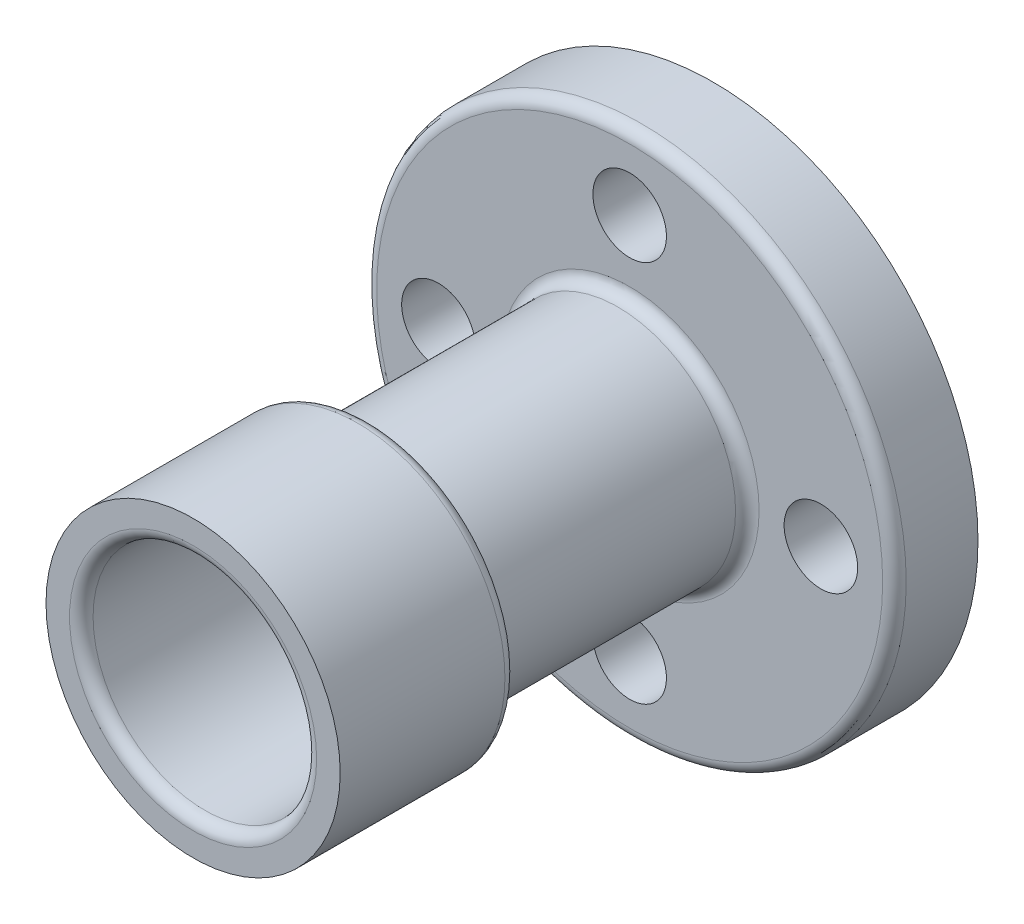
ISO-10303-21;
HEADER;
FILE_DESCRIPTION(('STEP AP214'),'2;1');
FILE_NAME('part.step','',(''),(''),'','','');
FILE_SCHEMA(('AUTOMOTIVE_DESIGN { 1 0 10303 214 1 1 1 1 }'));
ENDSEC;
DATA;
#1=APPLICATION_CONTEXT('core data for automotive mechanical design processes');
#2=APPLICATION_PROTOCOL_DEFINITION('international standard','automotive_design',2000,#1);
#3=PRODUCT_CONTEXT('',#1,'mechanical');
#4=PRODUCT('Part','Part','',(#3));
#5=PRODUCT_RELATED_PRODUCT_CATEGORY('part','',(#4));
#6=PRODUCT_DEFINITION_FORMATION('','',#4);
#7=PRODUCT_DEFINITION_CONTEXT('part definition',#1,'design');
#8=PRODUCT_DEFINITION('design','',#6,#7);
#9=PRODUCT_DEFINITION_SHAPE('','',#8);
#10=(LENGTH_UNIT() NAMED_UNIT(*) SI_UNIT(.MILLI.,.METRE.));
#11=(NAMED_UNIT(*) PLANE_ANGLE_UNIT() SI_UNIT($,.RADIAN.));
#12=(NAMED_UNIT(*) SI_UNIT($,.STERADIAN.) SOLID_ANGLE_UNIT());
#13=UNCERTAINTY_MEASURE_WITH_UNIT(LENGTH_MEASURE(1.E-05),#10,'distance_accuracy_value','');
#14=(GEOMETRIC_REPRESENTATION_CONTEXT(3) GLOBAL_UNCERTAINTY_ASSIGNED_CONTEXT((#13)) GLOBAL_UNIT_ASSIGNED_CONTEXT((#10,
#11,#12)) REPRESENTATION_CONTEXT('',''));
#15=CARTESIAN_POINT('',(0.,0.,0.));
#16=DIRECTION('',(0.,0.,1.));
#17=DIRECTION('',(1.,0.,0.));
#18=AXIS2_PLACEMENT_3D('',#15,#16,#17);
#19=CARTESIAN_POINT('',(0.,0.,58.4));
#20=DIRECTION('',(0.,0.,1.));
#21=DIRECTION('',(1.,0.,0.));
#22=AXIS2_PLACEMENT_3D('',#19,#20,#21);
#23=PLANE('',#22);
#24=CARTESIAN_POINT('',(0.,0.,58.4));
#25=DIRECTION('',(0.,0.,1.));
#26=DIRECTION('',(1.,0.,0.));
#27=AXIS2_PLACEMENT_3D('',#24,#25,#26);
#28=CIRCLE('',#27,17.);
#29=CARTESIAN_POINT('',(17.,0.,58.4));
#30=VERTEX_POINT('',#29);
#31=EDGE_CURVE('E53',#30,#30,#28,.F.);
#32=ORIENTED_EDGE('',*,*,#31,.T.);
#33=EDGE_LOOP('',(#32));
#34=FACE_BOUND('',#33,.T.);
#35=CARTESIAN_POINT('',(0.,0.,58.4));
#36=DIRECTION('',(0.,0.,1.));
#37=DIRECTION('',(1.,0.,0.));
#38=AXIS2_PLACEMENT_3D('',#35,#36,#37);
#39=CIRCLE('',#38,19.);
#40=CARTESIAN_POINT('',(19.,0.,58.4));
#41=VERTEX_POINT('',#40);
#42=EDGE_CURVE('E79',#41,#41,#39,.F.);
#43=ORIENTED_EDGE('',*,*,#42,.F.);
#44=EDGE_LOOP('',(#43));
#45=FACE_BOUND('',#44,.T.);
#46=ADVANCED_FACE('F39',(#34,#45),#23,.T.);
#47=CARTESIAN_POINT('',(0.,0.,14.2));
#48=DIRECTION('',(0.,0.,-1.));
#49=DIRECTION('',(-1.,0.,0.));
#50=AXIS2_PLACEMENT_3D('',#47,#48,#49);
#51=CYLINDRICAL_SURFACE('',#50,45.);
#52=CARTESIAN_POINT('',(0.,0.,12.2));
#53=DIRECTION('',(0.,0.,1.));
#54=DIRECTION('',(1.,0.,0.));
#55=AXIS2_PLACEMENT_3D('',#52,#53,#54);
#56=CIRCLE('',#55,45.);
#57=CARTESIAN_POINT('',(45.,0.,12.2));
#58=VERTEX_POINT('',#57);
#59=EDGE_CURVE('E72',#58,#58,#56,.F.);
#60=ORIENTED_EDGE('',*,*,#59,.T.);
#61=EDGE_LOOP('',(#60));
#62=FACE_BOUND('',#61,.T.);
#63=CARTESIAN_POINT('',(0.,0.,0.));
#64=DIRECTION('',(0.,0.,1.));
#65=DIRECTION('',(1.,0.,0.));
#66=AXIS2_PLACEMENT_3D('',#63,#64,#65);
#67=CIRCLE('',#66,45.);
#68=CARTESIAN_POINT('',(45.,0.,0.));
#69=VERTEX_POINT('',#68);
#70=EDGE_CURVE('E88',#69,#69,#67,.T.);
#71=ORIENTED_EDGE('',*,*,#70,.T.);
#72=EDGE_LOOP('',(#71));
#73=FACE_BOUND('',#72,.T.);
#74=ADVANCED_FACE('F136',(#62,#73),#51,.T.);
#75=CARTESIAN_POINT('',(0.,0.,14.2));
#76=DIRECTION('',(0.,0.,1.));
#77=DIRECTION('',(1.,0.,0.));
#78=AXIS2_PLACEMENT_3D('',#75,#76,#77);
#79=PLANE('',#78);
#80=CARTESIAN_POINT('',(0.,0.,14.2));
#81=DIRECTION('',(0.,0.,1.));
#82=DIRECTION('',(1.,0.,0.));
#83=AXIS2_PLACEMENT_3D('',#80,#81,#82);
#84=CIRCLE('',#83,22.);
#85=CARTESIAN_POINT('',(22.,0.,14.2));
#86=VERTEX_POINT('',#85);
#87=EDGE_CURVE('E63',#86,#86,#84,.F.);
#88=ORIENTED_EDGE('',*,*,#87,.T.);
#89=EDGE_LOOP('',(#88));
#90=FACE_BOUND('',#89,.T.);
#91=CARTESIAN_POINT('',(0.,0.,14.2));
#92=DIRECTION('',(0.,0.,1.));
#93=DIRECTION('',(1.,0.,0.));
#94=AXIS2_PLACEMENT_3D('',#91,#92,#93);
#95=CIRCLE('',#94,43.);
#96=CARTESIAN_POINT('',(43.,0.,14.2));
#97=VERTEX_POINT('',#96);
#98=EDGE_CURVE('E74',#97,#97,#95,.T.);
#99=ORIENTED_EDGE('',*,*,#98,.T.);
#100=EDGE_LOOP('',(#99));
#101=FACE_BOUND('',#100,.T.);
#102=CARTESIAN_POINT('',(0.,32.5,14.2));
#103=DIRECTION('',(0.,0.,1.));
#104=DIRECTION('',(1.,0.,0.));
#105=AXIS2_PLACEMENT_3D('',#102,#103,#104);
#106=CIRCLE('',#105,6.25);
#107=CARTESIAN_POINT('',(6.25,32.5,14.2));
#108=VERTEX_POINT('',#107);
#109=EDGE_CURVE('E108',#108,#108,#106,.T.);
#110=ORIENTED_EDGE('',*,*,#109,.F.);
#111=EDGE_LOOP('',(#110));
#112=FACE_BOUND('',#111,.T.);
#113=CARTESIAN_POINT('',(0.,-32.5,14.2));
#114=DIRECTION('',(0.,0.,1.));
#115=DIRECTION('',(1.,0.,0.));
#116=AXIS2_PLACEMENT_3D('',#113,#114,#115);
#117=CIRCLE('',#116,6.25);
#118=CARTESIAN_POINT('',(6.25,-32.5,14.2));
#119=VERTEX_POINT('',#118);
#120=EDGE_CURVE('E103',#119,#119,#117,.T.);
#121=ORIENTED_EDGE('',*,*,#120,.F.);
#122=EDGE_LOOP('',(#121));
#123=FACE_BOUND('',#122,.T.);
#124=CARTESIAN_POINT('',(-32.5,0.,14.2));
#125=DIRECTION('',(0.,0.,1.));
#126=DIRECTION('',(1.,0.,0.));
#127=AXIS2_PLACEMENT_3D('',#124,#125,#126);
#128=CIRCLE('',#127,6.25);
#129=CARTESIAN_POINT('',(-26.25,0.,14.2));
#130=VERTEX_POINT('',#129);
#131=EDGE_CURVE('E100',#130,#130,#128,.T.);
#132=ORIENTED_EDGE('',*,*,#131,.F.);
#133=EDGE_LOOP('',(#132));
#134=FACE_BOUND('',#133,.T.);
#135=CARTESIAN_POINT('',(32.5,0.,14.2));
#136=DIRECTION('',(0.,0.,1.));
#137=DIRECTION('',(1.,0.,0.));
#138=AXIS2_PLACEMENT_3D('',#135,#136,#137);
#139=CIRCLE('',#138,6.25);
#140=CARTESIAN_POINT('',(38.75,0.,14.2));
#141=VERTEX_POINT('',#140);
#142=EDGE_CURVE('E89',#141,#141,#139,.T.);
#143=ORIENTED_EDGE('',*,*,#142,.F.);
#144=EDGE_LOOP('',(#143));
#145=FACE_BOUND('',#144,.T.);
#146=ADVANCED_FACE('F148',(#90,#101,#112,#123,#134,#145),#79,.T.);
#147=CARTESIAN_POINT('',(0.,0.,0.));
#148=DIRECTION('',(0.,0.,1.));
#149=DIRECTION('',(1.,0.,0.));
#150=AXIS2_PLACEMENT_3D('',#147,#148,#149);
#151=PLANE('',#150);
#152=CARTESIAN_POINT('',(0.,0.,0.));
#153=DIRECTION('',(0.,0.,1.));
#154=DIRECTION('',(1.,0.,0.));
#155=AXIS2_PLACEMENT_3D('',#152,#153,#154);
#156=CIRCLE('',#155,18.0000000000002);
#157=CARTESIAN_POINT('',(-18.0000000000002,0.,0.));
#158=VERTEX_POINT('',#157);
#159=EDGE_CURVE('E78',#158,#158,#156,.T.);
#160=ORIENTED_EDGE('',*,*,#159,.T.);
#161=EDGE_LOOP('',(#160));
#162=FACE_BOUND('',#161,.T.);
#163=CARTESIAN_POINT('',(0.,32.5,0.));
#164=DIRECTION('',(0.,0.,1.));
#165=DIRECTION('',(1.,0.,0.));
#166=AXIS2_PLACEMENT_3D('',#163,#164,#165);
#167=CIRCLE('',#166,6.25);
#168=CARTESIAN_POINT('',(6.25,32.5,0.));
#169=VERTEX_POINT('',#168);
#170=EDGE_CURVE('E90',#169,#169,#167,.T.);
#171=ORIENTED_EDGE('',*,*,#170,.T.);
#172=EDGE_LOOP('',(#171));
#173=FACE_BOUND('',#172,.T.);
#174=CARTESIAN_POINT('',(0.,-32.5,0.));
#175=DIRECTION('',(0.,0.,1.));
#176=DIRECTION('',(1.,0.,0.));
#177=AXIS2_PLACEMENT_3D('',#174,#175,#176);
#178=CIRCLE('',#177,6.25);
#179=CARTESIAN_POINT('',(6.25,-32.5,0.));
#180=VERTEX_POINT('',#179);
#181=EDGE_CURVE('E106',#180,#180,#178,.T.);
#182=ORIENTED_EDGE('',*,*,#181,.T.);
#183=EDGE_LOOP('',(#182));
#184=FACE_BOUND('',#183,.T.);
#185=CARTESIAN_POINT('',(-32.5,0.,0.));
#186=DIRECTION('',(0.,0.,1.));
#187=DIRECTION('',(1.,0.,0.));
#188=AXIS2_PLACEMENT_3D('',#185,#186,#187);
#189=CIRCLE('',#188,6.25);
#190=CARTESIAN_POINT('',(-26.25,0.,0.));
#191=VERTEX_POINT('',#190);
#192=EDGE_CURVE('E99',#191,#191,#189,.T.);
#193=ORIENTED_EDGE('',*,*,#192,.T.);
#194=EDGE_LOOP('',(#193));
#195=FACE_BOUND('',#194,.T.);
#196=CARTESIAN_POINT('',(32.5,0.,0.));
#197=DIRECTION('',(0.,0.,1.));
#198=DIRECTION('',(1.,0.,0.));
#199=AXIS2_PLACEMENT_3D('',#196,#197,#198);
#200=CIRCLE('',#199,6.25);
#201=CARTESIAN_POINT('',(38.75,0.,0.));
#202=VERTEX_POINT('',#201);
#203=EDGE_CURVE('E91',#202,#202,#200,.T.);
#204=ORIENTED_EDGE('',*,*,#203,.T.);
#205=EDGE_LOOP('',(#204));
#206=FACE_BOUND('',#205,.T.);
#207=ORIENTED_EDGE('',*,*,#70,.F.);
#208=EDGE_LOOP('',(#207));
#209=FACE_BOUND('',#208,.T.);
#210=ADVANCED_FACE('F172',(#162,#173,#184,#195,#206,#209),#151,.F.);
#211=CARTESIAN_POINT('',(32.5,0.,0.));
#212=DIRECTION('',(0.,0.,1.));
#213=DIRECTION('',(1.,0.,0.));
#214=AXIS2_PLACEMENT_3D('',#211,#212,#213);
#215=CYLINDRICAL_SURFACE('',#214,6.25);
#216=ORIENTED_EDGE('',*,*,#203,.F.);
#217=EDGE_LOOP('',(#216));
#218=FACE_BOUND('',#217,.T.);
#219=ORIENTED_EDGE('',*,*,#142,.T.);
#220=EDGE_LOOP('',(#219));
#221=FACE_BOUND('',#220,.T.);
#222=ADVANCED_FACE('F170',(#218,#221),#215,.F.);
#223=CARTESIAN_POINT('',(-32.5,0.,0.));
#224=DIRECTION('',(0.,0.,1.));
#225=DIRECTION('',(1.,0.,0.));
#226=AXIS2_PLACEMENT_3D('',#223,#224,#225);
#227=CYLINDRICAL_SURFACE('',#226,6.25);
#228=ORIENTED_EDGE('',*,*,#192,.F.);
#229=EDGE_LOOP('',(#228));
#230=FACE_BOUND('',#229,.T.);
#231=ORIENTED_EDGE('',*,*,#131,.T.);
#232=EDGE_LOOP('',(#231));
#233=FACE_BOUND('',#232,.T.);
#234=ADVANCED_FACE('F162',(#230,#233),#227,.F.);
#235=CARTESIAN_POINT('',(0.,-32.5,0.));
#236=DIRECTION('',(0.,0.,1.));
#237=DIRECTION('',(1.,0.,0.));
#238=AXIS2_PLACEMENT_3D('',#235,#236,#237);
#239=CYLINDRICAL_SURFACE('',#238,6.25);
#240=ORIENTED_EDGE('',*,*,#181,.F.);
#241=EDGE_LOOP('',(#240));
#242=FACE_BOUND('',#241,.T.);
#243=ORIENTED_EDGE('',*,*,#120,.T.);
#244=EDGE_LOOP('',(#243));
#245=FACE_BOUND('',#244,.T.);
#246=ADVANCED_FACE('F157',(#242,#245),#239,.F.);
#247=CARTESIAN_POINT('',(0.,32.5,0.));
#248=DIRECTION('',(0.,0.,1.));
#249=DIRECTION('',(1.,0.,0.));
#250=AXIS2_PLACEMENT_3D('',#247,#248,#249);
#251=CYLINDRICAL_SURFACE('',#250,6.25);
#252=ORIENTED_EDGE('',*,*,#170,.F.);
#253=EDGE_LOOP('',(#252));
#254=FACE_BOUND('',#253,.T.);
#255=ORIENTED_EDGE('',*,*,#109,.T.);
#256=EDGE_LOOP('',(#255));
#257=FACE_BOUND('',#256,.T.);
#258=ADVANCED_FACE('F154',(#254,#257),#251,.F.);
#259=CARTESIAN_POINT('',(0.,0.,58.4));
#260=DIRECTION('',(0.,0.,-1.));
#261=DIRECTION('',(-1.,0.,0.));
#262=AXIS2_PLACEMENT_3D('',#259,#260,#261);
#263=CYLINDRICAL_SURFACE('',#262,20.);
#264=CARTESIAN_POINT('',(0.,0.,16.2));
#265=DIRECTION('',(0.,0.,1.));
#266=DIRECTION('',(1.,0.,0.));
#267=AXIS2_PLACEMENT_3D('',#264,#265,#266);
#268=CIRCLE('',#267,20.);
#269=CARTESIAN_POINT('',(20.,0.,16.2));
#270=VERTEX_POINT('',#269);
#271=EDGE_CURVE('E66',#270,#270,#268,.T.);
#272=ORIENTED_EDGE('',*,*,#271,.T.);
#273=EDGE_LOOP('',(#272));
#274=FACE_BOUND('',#273,.T.);
#275=CARTESIAN_POINT('',(0.,0.,58.4));
#276=DIRECTION('',(0.,0.,1.));
#277=DIRECTION('',(1.,0.,0.));
#278=AXIS2_PLACEMENT_3D('',#275,#276,#277);
#279=CIRCLE('',#278,20.);
#280=CARTESIAN_POINT('',(20.,0.,58.4));
#281=VERTEX_POINT('',#280);
#282=EDGE_CURVE('E94',#281,#281,#279,.T.);
#283=ORIENTED_EDGE('',*,*,#282,.F.);
#284=EDGE_LOOP('',(#283));
#285=FACE_BOUND('',#284,.T.);
#286=ADVANCED_FACE('F155',(#274,#285),#263,.T.);
#287=CARTESIAN_POINT('',(0.,0.,58.4));
#288=DIRECTION('',(0.,0.,-1.));
#289=DIRECTION('',(-1.,0.,0.));
#290=AXIS2_PLACEMENT_3D('',#287,#288,#289);
#291=CYLINDRICAL_SURFACE('',#290,15.);
#292=CARTESIAN_POINT('',(0.,0.,56.4));
#293=DIRECTION('',(0.,0.,1.));
#294=DIRECTION('',(1.,0.,0.));
#295=AXIS2_PLACEMENT_3D('',#292,#293,#294);
#296=CIRCLE('',#295,15.);
#297=CARTESIAN_POINT('',(15.,0.,56.4));
#298=VERTEX_POINT('',#297);
#299=EDGE_CURVE('E49',#298,#298,#296,.T.);
#300=ORIENTED_EDGE('',*,*,#299,.T.);
#301=EDGE_LOOP('',(#300));
#302=FACE_BOUND('',#301,.T.);
#303=CARTESIAN_POINT('',(0.,0.,0.183487860451456));
#304=DIRECTION('',(0.,0.,1.));
#305=DIRECTION('',(1.,0.,0.));
#306=AXIS2_PLACEMENT_3D('',#303,#304,#305);
#307=CIRCLE('',#306,15.);
#308=CARTESIAN_POINT('',(-15.,0.,0.183487860451456));
#309=VERTEX_POINT('',#308);
#310=EDGE_CURVE('E81',#309,#309,#307,.F.);
#311=ORIENTED_EDGE('',*,*,#310,.T.);
#312=EDGE_LOOP('',(#311));
#313=FACE_BOUND('',#312,.T.);
#314=ADVANCED_FACE('F151',(#302,#313),#291,.F.);
#315=CARTESIAN_POINT('',(0.,0.,0.183487860451456));
#316=DIRECTION('',(0.,0.,-1.));
#317=DIRECTION('',(-1.,0.,0.));
#318=AXIS2_PLACEMENT_3D('',#315,#316,#317);
#319=CONICAL_SURFACE('',#318,15.,1.5097098029751);
#320=CARTESIAN_POINT('',(-18.0000000000002,0.,0.));
#321=CARTESIAN_POINT('',(-17.9687500000002,0.,0.00191133187970259));
#322=CARTESIAN_POINT('',(-17.9375000000002,0.,0.00382266375940528));
#323=CARTESIAN_POINT('',(-17.8750000000002,0.,0.00764532751881067));
#324=CARTESIAN_POINT('',(-17.8437500000001,0.,0.00955665939851337));
#325=CARTESIAN_POINT('',(-17.7812500000001,0.,0.0133793231579187));
#326=CARTESIAN_POINT('',(-17.7500000000001,0.,0.0152906550376213));
#327=CARTESIAN_POINT('',(-17.6875000000001,0.,0.0191133187970266));
#328=CARTESIAN_POINT('',(-17.6562500000001,0.,0.0210246506767294));
#329=CARTESIAN_POINT('',(-17.5937500000001,0.,0.0248473144361347));
#330=CARTESIAN_POINT('',(-17.5625000000001,0.,0.0267586463158373));
#331=CARTESIAN_POINT('',(-17.5000000000001,0.,0.0305813100752426));
#332=CARTESIAN_POINT('',(-17.4687500000001,0.,0.0324926419549453));
#333=CARTESIAN_POINT('',(-17.4062500000001,0.,0.0363153057143507));
#334=CARTESIAN_POINT('',(-17.3750000000001,0.,0.0382266375940534));
#335=CARTESIAN_POINT('',(-17.3125000000001,0.,0.0420493013534587));
#336=CARTESIAN_POINT('',(-17.2812500000001,0.,0.0439606332331613));
#337=CARTESIAN_POINT('',(-17.2187500000001,0.,0.0477832969925666));
#338=CARTESIAN_POINT('',(-17.1875000000001,0.,0.0496946288722694));
#339=CARTESIAN_POINT('',(-17.1250000000001,0.,0.0535172926316747));
#340=CARTESIAN_POINT('',(-17.0937500000001,0.,0.0554286245113773));
#341=CARTESIAN_POINT('',(-17.0312500000001,0.,0.0592512882707826));
#342=CARTESIAN_POINT('',(-17.0000000000001,0.,0.0611626201504853));
#343=CARTESIAN_POINT('',(-16.9375000000001,0.,0.0649852839098907));
#344=CARTESIAN_POINT('',(-16.9062500000001,0.,0.0668966157895934));
#345=CARTESIAN_POINT('',(-16.8437500000001,0.,0.0707192795489987));
#346=CARTESIAN_POINT('',(-16.8125000000001,0.,0.0726306114287013));
#347=CARTESIAN_POINT('',(-16.7500000000001,0.,0.0764532751881067));
#348=CARTESIAN_POINT('',(-16.7187500000001,0.,0.0783646070678094));
#349=CARTESIAN_POINT('',(-16.6562500000001,0.,0.0821872708272148));
#350=CARTESIAN_POINT('',(-16.6250000000001,0.,0.0840986027069174));
#351=CARTESIAN_POINT('',(-16.5625000000001,0.,0.0879212664663227));
#352=CARTESIAN_POINT('',(-16.5312500000001,0.,0.0898325983460254));
#353=CARTESIAN_POINT('',(-16.4687500000001,0.,0.0936552621054308));
#354=CARTESIAN_POINT('',(-16.4375000000001,0.,0.0955665939851334));
#355=CARTESIAN_POINT('',(-16.3750000000001,0.,0.0993892577445388));
#356=CARTESIAN_POINT('',(-16.3437500000001,0.,0.101300589624241));
#357=CARTESIAN_POINT('',(-16.2812500000001,0.,0.105123253383647));
#358=CARTESIAN_POINT('',(-16.2500000000001,0.,0.107034585263349));
#359=CARTESIAN_POINT('',(-16.1875000000001,0.,0.110857249022755));
#360=CARTESIAN_POINT('',(-16.1562500000001,0.,0.112768580902457));
#361=CARTESIAN_POINT('',(-16.0937500000001,0.,0.116591244661863));
#362=CARTESIAN_POINT('',(-16.0625000000001,0.,0.118502576541565));
#363=CARTESIAN_POINT('',(-16.0000000000001,0.,0.122325240300971));
#364=CARTESIAN_POINT('',(-15.96875,0.,0.124236572180673));
#365=CARTESIAN_POINT('',(-15.90625,0.,0.128059235940079));
#366=CARTESIAN_POINT('',(-15.875,0.,0.129970567819781));
#367=CARTESIAN_POINT('',(-15.8125,0.,0.133793231579187));
#368=CARTESIAN_POINT('',(-15.78125,0.,0.135704563458889));
#369=CARTESIAN_POINT('',(-15.71875,0.,0.139527227218295));
#370=CARTESIAN_POINT('',(-15.6875,0.,0.141438559097997));
#371=CARTESIAN_POINT('',(-15.625,0.,0.145261222857403));
#372=CARTESIAN_POINT('',(-15.59375,0.,0.147172554737105));
#373=CARTESIAN_POINT('',(-15.53125,0.,0.150995218496511));
#374=CARTESIAN_POINT('',(-15.5,0.,0.152906550376213));
#375=CARTESIAN_POINT('',(-15.4375,0.,0.156729214135619));
#376=CARTESIAN_POINT('',(-15.40625,0.,0.158640546015321));
#377=CARTESIAN_POINT('',(-15.34375,0.,0.162463209774727));
#378=CARTESIAN_POINT('',(-15.3125,0.,0.164374541654429));
#379=CARTESIAN_POINT('',(-15.25,0.,0.168197205413835));
#380=CARTESIAN_POINT('',(-15.21875,0.,0.170108537293538));
#381=CARTESIAN_POINT('',(-15.15625,0.,0.173931201052943));
#382=CARTESIAN_POINT('',(-15.125,0.,0.175842532932645));
#383=CARTESIAN_POINT('',(-15.0625,0.,0.179665196692051));
#384=CARTESIAN_POINT('',(-15.03125,0.,0.181576528571753));
#385=CARTESIAN_POINT('',(-15.,0.,0.183487860451456));
#386=B_SPLINE_CURVE_WITH_KNOTS('',3,(#320,#321,#322,#323,#324,#325,#326,#327,#328,#329,#330,
#331,#332,#333,#334,#335,#336,#337,#338,#339,#340,#341,#342,#343,#344,#345,#346,#347,#348,#349,
#350,#351,#352,#353,#354,#355,#356,#357,#358,#359,#360,#361,#362,#363,#364,#365,#366,#367,#368,
#369,#370,#371,#372,#373,#374,#375,#376,#377,#378,#379,#380,#381,#382,#383,#384,#385),
.UNSPECIFIED.,.F.,.F.,(4,2,2,2,2,2,2,2,2,2,2,2,2,2,2,2,2,2,2,2,2,2,2,2,2,2,2,2,2,2,2,2,4),(0.,
0.0939251894115204,0.187850378823041,0.281775568234565,0.375700757646085,0.469625947057609,
0.563551136469129,0.657476325880649,0.751401515292173,0.845326704703694,0.939251894115217,
1.03317708352674,1.12710227293826,1.22102746234978,1.3149526517613,1.40887784117283,
1.50280303058435,1.59672821999587,1.69065340940739,1.78457859881891,1.87850378823043,
1.97242897764196,2.06635416705348,2.160279356465,2.25420454587652,2.34812973528804,
2.44205492469956,2.53598011411108,2.62990530352261,2.72383049293413,2.81775568234565,
2.91168087175717,3.00560606116869),.UNSPECIFIED.);
#387=EDGE_CURVE('BSEAM177',#158,#309,#386,.T.);
#388=ORIENTED_EDGE('',*,*,#159,.F.);
#389=ORIENTED_EDGE('',*,*,#310,.F.);
#390=ORIENTED_EDGE('',*,*,#387,.T.);
#391=ORIENTED_EDGE('',*,*,#387,.F.);
#392=EDGE_LOOP('',(#388,#390,#389,#391));
#393=FACE_BOUND('',#392,.T.);
#394=ADVANCED_FACE('F177',(#393),#319,.F.);
#395=CARTESIAN_POINT('',(0.,0.,88.4));
#396=DIRECTION('',(0.,0.,1.));
#397=DIRECTION('',(1.,0.,0.));
#398=AXIS2_PLACEMENT_3D('',#395,#396,#397);
#399=PLANE('',#398);
#400=CARTESIAN_POINT('',(0.,0.,88.4));
#401=DIRECTION('',(0.,0.,1.));
#402=DIRECTION('',(1.,0.,0.));
#403=AXIS2_PLACEMENT_3D('',#400,#401,#402);
#404=CIRCLE('',#403,21.);
#405=CARTESIAN_POINT('',(21.,0.,88.4));
#406=VERTEX_POINT('',#405);
#407=EDGE_CURVE('E56',#406,#406,#404,.F.);
#408=ORIENTED_EDGE('',*,*,#407,.T.);
#409=EDGE_LOOP('',(#408));
#410=FACE_BOUND('',#409,.T.);
#411=CARTESIAN_POINT('',(0.,0.,88.4));
#412=DIRECTION('',(0.,0.,1.));
#413=DIRECTION('',(1.,0.,0.));
#414=AXIS2_PLACEMENT_3D('',#411,#412,#413);
#415=CIRCLE('',#414,25.);
#416=CARTESIAN_POINT('',(25.,0.,88.4));
#417=VERTEX_POINT('',#416);
#418=EDGE_CURVE('E117',#417,#417,#415,.T.);
#419=ORIENTED_EDGE('',*,*,#418,.T.);
#420=EDGE_LOOP('',(#419));
#421=FACE_BOUND('',#420,.T.);
#422=ADVANCED_FACE('F118',(#410,#421),#399,.T.);
#423=CARTESIAN_POINT('',(0.,0.,58.4));
#424=DIRECTION('',(0.,0.,1.));
#425=DIRECTION('',(1.,0.,0.));
#426=AXIS2_PLACEMENT_3D('',#423,#424,#425);
#427=PLANE('',#426);
#428=CARTESIAN_POINT('',(0.,0.,58.4));
#429=DIRECTION('',(0.,0.,1.));
#430=DIRECTION('',(1.,0.,0.));
#431=AXIS2_PLACEMENT_3D('',#428,#429,#430);
#432=CIRCLE('',#431,23.);
#433=CARTESIAN_POINT('',(23.,0.,58.4));
#434=VERTEX_POINT('',#433);
#435=EDGE_CURVE('E10',#434,#434,#432,.F.);
#436=ORIENTED_EDGE('',*,*,#435,.T.);
#437=EDGE_LOOP('',(#436));
#438=FACE_BOUND('',#437,.T.);
#439=ORIENTED_EDGE('',*,*,#282,.T.);
#440=EDGE_LOOP('',(#439));
#441=FACE_BOUND('',#440,.T.);
#442=ADVANCED_FACE('F122',(#438,#441),#427,.F.);
#443=CARTESIAN_POINT('',(0.,0.,88.4));
#444=DIRECTION('',(0.,0.,-1.));
#445=DIRECTION('',(-1.,0.,0.));
#446=AXIS2_PLACEMENT_3D('',#443,#444,#445);
#447=CYLINDRICAL_SURFACE('',#446,25.);
#448=CARTESIAN_POINT('',(0.,0.,60.4));
#449=DIRECTION('',(0.,0.,1.));
#450=DIRECTION('',(1.,0.,0.));
#451=AXIS2_PLACEMENT_3D('',#448,#449,#450);
#452=CIRCLE('',#451,25.);
#453=CARTESIAN_POINT('',(25.,0.,60.4));
#454=VERTEX_POINT('',#453);
#455=EDGE_CURVE('E46',#454,#454,#452,.T.);
#456=ORIENTED_EDGE('',*,*,#455,.T.);
#457=EDGE_LOOP('',(#456));
#458=FACE_BOUND('',#457,.T.);
#459=ORIENTED_EDGE('',*,*,#418,.F.);
#460=EDGE_LOOP('',(#459));
#461=FACE_BOUND('',#460,.T.);
#462=ADVANCED_FACE('F125',(#458,#461),#447,.T.);
#463=CARTESIAN_POINT('',(0.,0.,88.4));
#464=DIRECTION('',(0.,0.,-1.));
#465=DIRECTION('',(-1.,0.,0.));
#466=AXIS2_PLACEMENT_3D('',#463,#464,#465);
#467=CYLINDRICAL_SURFACE('',#466,19.);
#468=CARTESIAN_POINT('',(0.,0.,86.4));
#469=DIRECTION('',(0.,0.,1.));
#470=DIRECTION('',(1.,0.,0.));
#471=AXIS2_PLACEMENT_3D('',#468,#469,#470);
#472=CIRCLE('',#471,19.);
#473=CARTESIAN_POINT('',(19.,0.,86.4));
#474=VERTEX_POINT('',#473);
#475=EDGE_CURVE('E64',#474,#474,#472,.T.);
#476=ORIENTED_EDGE('',*,*,#475,.T.);
#477=EDGE_LOOP('',(#476));
#478=FACE_BOUND('',#477,.T.);
#479=ORIENTED_EDGE('',*,*,#42,.T.);
#480=EDGE_LOOP('',(#479));
#481=FACE_BOUND('',#480,.T.);
#482=ADVANCED_FACE('F124',(#478,#481),#467,.F.);
#483=CARTESIAN_POINT('',(0.,0.,12.2));
#484=DIRECTION('',(0.,0.,1.));
#485=DIRECTION('',(1.,0.,0.));
#486=AXIS2_PLACEMENT_3D('',#483,#484,#485);
#487=TOROIDAL_SURFACE('',#486,43.,2.);
#488=ORIENTED_EDGE('',*,*,#59,.F.);
#489=EDGE_LOOP('',(#488));
#490=FACE_BOUND('',#489,.T.);
#491=ORIENTED_EDGE('',*,*,#98,.F.);
#492=EDGE_LOOP('',(#491));
#493=FACE_BOUND('',#492,.T.);
#494=ADVANCED_FACE('F134',(#490,#493),#487,.T.);
#495=CARTESIAN_POINT('',(0.,0.,16.2));
#496=DIRECTION('',(0.,0.,1.));
#497=DIRECTION('',(1.,0.,0.));
#498=AXIS2_PLACEMENT_3D('',#495,#496,#497);
#499=TOROIDAL_SURFACE('',#498,22.,2.);
#500=ORIENTED_EDGE('',*,*,#87,.F.);
#501=EDGE_LOOP('',(#500));
#502=FACE_BOUND('',#501,.T.);
#503=ORIENTED_EDGE('',*,*,#271,.F.);
#504=EDGE_LOOP('',(#503));
#505=FACE_BOUND('',#504,.T.);
#506=ADVANCED_FACE('F190',(#502,#505),#499,.F.);
#507=CARTESIAN_POINT('',(0.,0.,86.4));
#508=DIRECTION('',(0.,0.,1.));
#509=DIRECTION('',(1.,0.,0.));
#510=AXIS2_PLACEMENT_3D('',#507,#508,#509);
#511=TOROIDAL_SURFACE('',#510,21.,2.);
#512=ORIENTED_EDGE('',*,*,#407,.F.);
#513=EDGE_LOOP('',(#512));
#514=FACE_BOUND('',#513,.T.);
#515=ORIENTED_EDGE('',*,*,#475,.F.);
#516=EDGE_LOOP('',(#515));
#517=FACE_BOUND('',#516,.T.);
#518=ADVANCED_FACE('F195',(#514,#517),#511,.T.);
#519=CARTESIAN_POINT('',(0.,0.,56.4));
#520=DIRECTION('',(0.,0.,1.));
#521=DIRECTION('',(1.,0.,0.));
#522=AXIS2_PLACEMENT_3D('',#519,#520,#521);
#523=TOROIDAL_SURFACE('',#522,17.,2.);
#524=ORIENTED_EDGE('',*,*,#299,.F.);
#525=EDGE_LOOP('',(#524));
#526=FACE_BOUND('',#525,.T.);
#527=ORIENTED_EDGE('',*,*,#31,.F.);
#528=EDGE_LOOP('',(#527));
#529=FACE_BOUND('',#528,.T.);
#530=ADVANCED_FACE('F194',(#526,#529),#523,.T.);
#531=CARTESIAN_POINT('',(0.,0.,60.4));
#532=DIRECTION('',(0.,0.,1.));
#533=DIRECTION('',(1.,0.,0.));
#534=AXIS2_PLACEMENT_3D('',#531,#532,#533);
#535=TOROIDAL_SURFACE('',#534,23.,2.);
#536=ORIENTED_EDGE('',*,*,#435,.F.);
#537=EDGE_LOOP('',(#536));
#538=FACE_BOUND('',#537,.T.);
#539=ORIENTED_EDGE('',*,*,#455,.F.);
#540=EDGE_LOOP('',(#539));
#541=FACE_BOUND('',#540,.T.);
#542=ADVANCED_FACE('F41',(#538,#541),#535,.T.);
#543=CLOSED_SHELL('',(#46,#74,#146,#210,#222,#234,#246,#258,#286,#314,#394,#422,#442,#462,#482,
#494,#506,#518,#530,#542));
#544=MANIFOLD_SOLID_BREP('B2',#543);
#545=ADVANCED_BREP_SHAPE_REPRESENTATION('',(#18,#544),#14);
#546=SHAPE_DEFINITION_REPRESENTATION(#9,#545);
ENDSEC;
END-ISO-10303-21;
